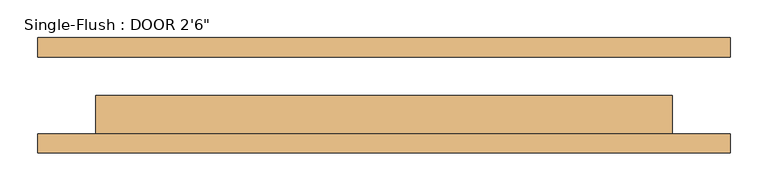
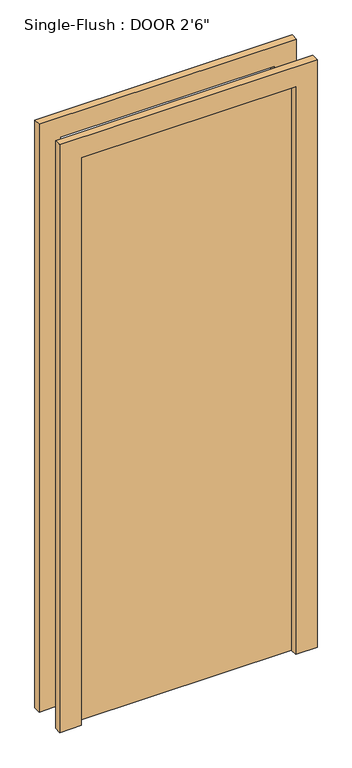
"""IFC4 building model written with IfcOpenShell, lengths in millimetres: door geometry."""

from ifc_helpers import new_model, si_unit, frame, origin, origin_with_axes, place, context, project, spatial, polyline, outline, extrude, source, transform, mapped, element, save


def door_aa9e95e7(model_context):
    return source(origin(), model_context, "Body", "SweptSolid", [
        extrude(outline(polyline([(2209.8, -457.2), (0.0, -457.2), (0.0, -381.0), (2133.6, -381.0), (2133.6, 381.0), (0.0, 381.0), (0.0, 457.2), (2209.8, 457.2), (2209.8, -457.2)])), frame((0.0, -76.2, 0.0), z_axis=(0.0, 1.0, 0.0), x_axis=(0.0, 0.0, 1.0)), (0.0, 0.0, 1.0), 25.4),
        extrude(outline(polyline([(2209.8, 457.2), (2209.8, -457.2), (0.0, -457.2), (0.0, -381.0), (2133.6, -381.0), (2133.6, 381.0), (0.0, 381.0), (0.0, 457.2), (2209.8, 457.2)])), frame((0.0, 50.8, 0.0), z_axis=(0.0, 1.0, 0.0), x_axis=(0.0, 0.0, 1.0)), (0.0, 0.0, 1.0), 25.4),
        extrude(outline(polyline([(381.0, 0.0), (381.0, -50.8), (-381.0, -50.8), (-381.0, 0.0), (381.0, 0.0)])), origin_with_axes(), (0.0, 0.0, 1.0), 2133.6),
    ])


if __name__ == "__main__":
    model = new_model("IFC4")
    model_context = context("Model", 3, world=origin())
    ifc_project = project(units=[si_unit("LENGTHUNIT", "METRE", prefix="MILLI")], contexts=[model_context])
    site = spatial("IfcSite", under=ifc_project)
    building = spatial("IfcBuilding", under=site)
    placement = place(None, origin())
    door_shape = door_aa9e95e7(model_context)
    element("IfcDoor", 1, ObjectType="Single-Flush : DOOR 2'6\"", at=placement, inside=building, context=model_context, shape_type="MappedRepresentation", body=[
        mapped(door_shape, transform((0.0, 0.0, 0.0), x_axis=(1.0, 0.0, 0.0), y_axis=(0.0, 1.0, 0.0), z_axis=(0.0, 0.0, 1.0))),
    ])
    save(model, "model.ifc")

# Revit data of these elements
# Type "Single-Flush : DOOR 2'6\""
#   Type Mark = "9"
#   Construction Type Id = "MDOOR"
#   Assembly Code = "C1020"
#   Analytic Construction = "Metal"
#   Thickness = 0' - 2"
#   Heat Transfer Coefficient (U) = 0.651978 BTU/(h·ft²·°F)
#   Height = 7' - 0"
#   Trim Projection Ext = 0' - 1"
#   Trim Projection Int = 0' - 1"
#   Trim Width = 0' - 3"
#   Width = 2' - 6"
#   Define Thermal Properties by = 1
#   Door Material = Door - Panel
#   Frame Material = Door - Frame
#   Visual Light Transmittance = 0
#   Solar Heat Gain Coefficient = 0
#   Function = (empty or 0)
#   Wall Closure = (empty or 0)
# Element 1 (IfcDoor, "Single-Flush : DOOR 2'6\"")
#   Materials on its faces: "Door - Frame", "Door - Panel"
# Materials
#   "Door - Panel": class "Wood", colour RGB 210 159 95, transparency 0, Cost = 0
#   "Door - Frame": colour RGB 118 70 51, transparency 0, Cost = 0
